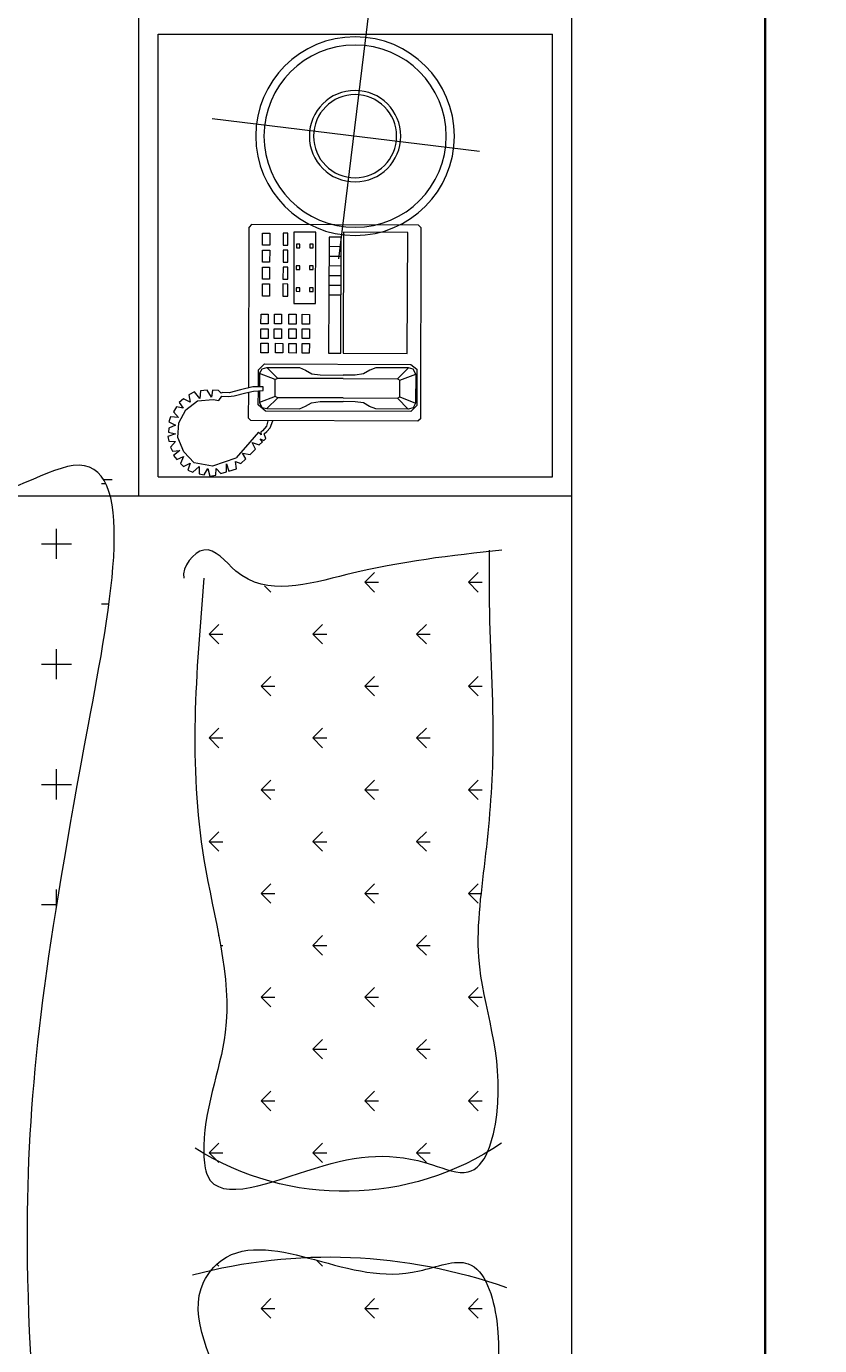
# Model space of a CAD drawing. Units: inches. Extents: x 3731 to 4318, y 1310 to 2388.
# Tile 20 of 57: x 4203 to 4237, y 1445 to 1502. Entities that reach past the tile are written whole.
import ezdxf

# ---------------------------------------------------------------- set-up
doc = ezdxf.new("R2010")
doc.units = ezdxf.units.IN
for name, color, linetype, lineweight in [('A-ANNO-DIMS', 2, 'Continuous', 18), ('A-FURN', 8, 'Continuous', 13), ('A-WALL', 7, 'Continuous', 35)]:
    doc.layers.add(name, color=color, linetype=linetype, lineweight=lineweight)
doc.styles.get("Standard").update_dxf_attribs({"font": 'arial.ttf'})
doc.dimstyles.get("Standard").update_dxf_attribs({"dimtxt": 0.18, "dimasz": 0.18, "dimexe": 0.18, "dimexo": 0.0625, "dimgap": 0.09, "dimtad": 0, "dimtih": 1, "dimtoh": 1, "dimdec": 4, "dimzin": 0, "dimdsep": 46, "dimtxsty": 'Standard', "dimcen": 0.09, "dimadec": 0, "dimazin": 0, "dimtfac": 1, "dimtdec": 4, "dimtofl": 0, "dimtmove": 0, "dimatfit": 3, "dimfxl": 1, "dimtolj": 1, "dimtzin": 0, "dimarcsym": 0})

# ---------------------------------------------------------------- blocks, each defined once
blk = doc.blocks.new('A$C200C7901')
for p, q in [((0.5, 2.3334), (2, 2.3334)), ((2, 2.3334), (2.5, 2.3334)), ((2, 1.6055), (2, 2.3334)), ((1.3176, 2.1721), (1.3075, 2.1822)), ((1.3176, 2.1721), (1.3075, 2.1822)), ((1.206, 2.0681), (1.1997, 2.0744)), ((1.206, 2.0681), (1.1997, 2.0744)), ((1.2019, 1.9645), (1.1997, 1.9666)), ((1.2019, 1.9645), (1.1997, 1.9666)), ((2, 1.8834), (2.5, 1.8834)), ((2.0171, 1.8467), (2.0171, 1.8556)), ((2.0171, 1.8467), (2.0171, 1.8556)), ((2.0129, 1.8445), (2.0129, 1.849)), ((2.0129, 1.8445), (2.0129, 1.849))]:
    blk.add_line(p, q)
at = {"linetype": 'ByBlock'}
for p, q in [((2.02, 2.3134), (2.48, 2.3134)), ((2.02, 1.9034), (2.02, 2.3134)), ((2.48, 1.9034), (2.48, 2.3134)), ((1.1559, 2.2259), (1.1458, 2.236)), ((1.1559, 2.2259), (1.1458, 2.236)), ((1.1559, 2.2259), (1.1559, 2.2402)), ((1.1559, 2.2259), (1.1559, 2.2402)), ((1.1559, 2.2259), (1.166, 2.236)), ((1.1559, 2.2259), (1.166, 2.236)), ((1.3714, 2.2259), (1.3613, 2.236)), ((1.3714, 2.2259), (1.3613, 2.236)), ((1.3714, 2.2259), (1.3714, 2.2402)), ((1.3714, 2.2259), (1.3714, 2.2402)), ((1.3714, 2.2259), (1.3815, 2.236)), ((1.3714, 2.2259), (1.3815, 2.236)), ((1.4792, 2.2259), (1.4691, 2.236)), ((1.4792, 2.2259), (1.4691, 2.236)), ((1.4792, 2.2259), (1.4792, 2.2402)), ((1.4792, 2.2259), (1.4792, 2.2402)), ((1.4792, 2.2259), (1.4893, 2.236)), ((1.4792, 2.2259), (1.4893, 2.236)), ((1.587, 2.2259), (1.5769, 2.236)), ((1.587, 2.2259), (1.5769, 2.236)), ((1.587, 2.2259), (1.587, 2.2393)), ((1.587, 2.2259), (1.587, 2.2393)), ((1.587, 2.2259), (1.5971, 2.236)), ((1.587, 2.2259), (1.5971, 2.236)), ((1.6947, 2.2259), (1.6846, 2.236)), ((1.6947, 2.2259), (1.6846, 2.236)), ((1.6947, 2.2259), (1.6947, 2.2402)), ((1.6947, 2.2259), (1.6947, 2.2402)), ((1.6947, 2.2259), (1.7048, 2.236)), ((1.6947, 2.2259), (1.7048, 2.236)), ((1.8025, 2.2259), (1.7924, 2.236)), ((1.8025, 2.2259), (1.7924, 2.236)), ((1.8025, 2.2259), (1.8025, 2.2402)), ((1.8025, 2.2259), (1.8025, 2.2402)), ((1.8025, 2.2259), (1.8126, 2.236)), ((1.8025, 2.2259), (1.8126, 2.236)), ((1.9103, 2.2259), (1.9002, 2.236)), ((1.9103, 2.2259), (1.9002, 2.236)), ((1.9103, 2.2259), (1.9103, 2.2402)), ((1.9103, 2.2259), (1.9103, 2.2402)), ((1.9103, 2.2259), (1.9204, 2.236)), ((1.9103, 2.2259), (1.9204, 2.236)), ((2.3581, 2.2373), (2.3919, 1.9595)), ((1.3176, 2.172), (1.3176, 2.1863)), ((1.3176, 2.172), (1.3176, 2.1863)), ((1.3176, 2.1721), (1.3277, 2.1822)), ((1.3176, 2.1721), (1.3277, 2.1822)), ((1.4253, 2.1721), (1.4152, 2.1822)), ((1.4253, 2.1721), (1.4152, 2.1822)), ((1.4253, 2.172), (1.4253, 2.1863)), ((1.4253, 2.172), (1.4253, 2.1863)), ((1.4253, 2.1721), (1.4354, 2.1822)), ((1.4253, 2.1721), (1.4354, 2.1822)), ((1.5331, 2.1721), (1.523, 2.1822)), ((1.5331, 2.1721), (1.523, 2.1822)), ((1.5331, 2.172), (1.5331, 2.1863)), ((1.5331, 2.172), (1.5331, 2.1863)), ((1.5331, 2.1721), (1.5432, 2.1822)), ((1.5331, 2.1721), (1.5432, 2.1822)), ((1.6409, 2.1721), (1.6308, 2.1822)), ((1.6409, 2.1721), (1.6308, 2.1822)), ((1.6408, 2.172), (1.6408, 2.1863)), ((1.6408, 2.172), (1.6408, 2.1863)), ((1.6409, 2.1721), (1.651, 2.1822)), ((1.6409, 2.1721), (1.651, 2.1822)), ((1.7486, 2.1721), (1.7385, 2.1822)), ((1.7486, 2.1721), (1.7385, 2.1822)), ((1.7486, 2.172), (1.7486, 2.1863)), ((1.7486, 2.172), (1.7486, 2.1863)), ((1.7486, 2.1721), (1.7587, 2.1822)), ((1.7486, 2.1721), (1.7587, 2.1822)), ((1.8564, 2.1721), (1.8463, 2.1822)), ((1.8564, 2.1721), (1.8463, 2.1822)), ((1.8564, 2.172), (1.8564, 2.1863)), ((1.8564, 2.172), (1.8564, 2.1863)), ((1.8564, 2.1721), (1.8665, 2.1822)), ((1.8564, 2.1721), (1.8665, 2.1822)), ((2.0802, 2.176), (2.0777, 2.1734)), ((2.0777, 2.1734), (2.0783, 1.9999)), ((2.2789, 2.1766), (2.0802, 2.176)), ((2.0941, 2.1722), (2.0878, 2.1659)), ((2.0878, 2.1659), (2.0883, 2.015)), ((2.0915, 2.1685), (2.0903, 2.1634)), ((2.0966, 2.171), (2.0915, 2.1685)), ((2.1318, 2.1724), (2.0941, 2.1722)), ((2.1267, 2.1711), (2.0966, 2.171)), ((2.1029, 2.1547), (2.0966, 2.171)), ((2.1205, 2.1547), (2.1267, 2.1711)), ((2.1267, 2.1711), (2.1318, 2.1686)), ((2.1368, 2.1661), (2.1318, 2.1724)), ((2.1318, 2.1686), (2.1331, 2.1636)), ((2.1373, 2.014), (2.1368, 2.1661)), ((2.2789, 2.1766), (2.2814, 2.1741)), ((2.2814, 2.1741), (2.282, 2.0006)), ((2.0903, 2.1634), (2.1017, 2.1521)), ((2.0903, 2.1634), (2.0904, 2.1295)), ((2.1017, 2.1521), (2.1029, 2.1547)), ((2.1019, 2.0956), (2.1017, 2.1521)), ((2.1029, 2.1547), (2.1205, 2.1547)), ((2.1218, 2.1522), (2.1205, 2.1547)), ((2.1331, 2.1636), (2.1218, 2.1522)), ((2.122, 2.0956), (2.1218, 2.1522)), ((2.1331, 2.1636), (2.1332, 2.1296)), ((2.1481, 2.1624), (2.2739, 2.1628)), ((2.1484, 2.0957), (2.1481, 2.1624)), ((2.2739, 2.1628), (2.2741, 2.0961)), ((1.1559, 2.1182), (1.1458, 2.1283)), ((1.1559, 2.1182), (1.1458, 2.1283)), ((1.1559, 2.1182), (1.1559, 2.1325)), ((1.1559, 2.1182), (1.1559, 2.1325)), ((1.1559, 2.1182), (1.166, 2.1283)), ((1.1559, 2.1182), (1.166, 2.1283)), ((1.3714, 2.1182), (1.3613, 2.1283)), ((1.3714, 2.1182), (1.3613, 2.1283)), ((1.3714, 2.1182), (1.3714, 2.1325)), ((1.3714, 2.1182), (1.3714, 2.1325)), ((1.3714, 2.1182), (1.3815, 2.1283)), ((1.3714, 2.1182), (1.3815, 2.1283)), ((1.4792, 2.1182), (1.4691, 2.1283)), ((1.4792, 2.1182), (1.4691, 2.1283)), ((1.4792, 2.1182), (1.4792, 2.1325)), ((1.4792, 2.1182), (1.4792, 2.1325)), ((1.4792, 2.1182), (1.4893, 2.1283)), ((1.4792, 2.1182), (1.4893, 2.1283)), ((1.587, 2.1182), (1.5769, 2.1283)), ((1.587, 2.1182), (1.5769, 2.1283)), ((1.587, 2.1182), (1.587, 2.1325)), ((1.587, 2.1182), (1.587, 2.1325)), ((1.587, 2.1182), (1.5971, 2.1283)), ((1.587, 2.1182), (1.5971, 2.1283)), ((1.6947, 2.1182), (1.6846, 2.1283)), ((1.6947, 2.1182), (1.6846, 2.1283)), ((1.6947, 2.1182), (1.6947, 2.1325)), ((1.6947, 2.1182), (1.6947, 2.1325)), ((1.6947, 2.1182), (1.7048, 2.1283)), ((1.6947, 2.1182), (1.7048, 2.1283)), ((1.8025, 2.1182), (1.7924, 2.1283)), ((1.8025, 2.1182), (1.7924, 2.1283)), ((1.8025, 2.1182), (1.8025, 2.1325)), ((1.8025, 2.1182), (1.8025, 2.1325)), ((1.8025, 2.1182), (1.8126, 2.1283)), ((1.8025, 2.1182), (1.8126, 2.1283)), ((1.9103, 2.1182), (1.9002, 2.1283)), ((1.9103, 2.1182), (1.9002, 2.1283)), ((1.9103, 2.1182), (1.9103, 2.1325)), ((1.9103, 2.1182), (1.9103, 2.1325)), ((1.9103, 2.1182), (1.9204, 2.1283)), ((1.9103, 2.1182), (1.9204, 2.1283)), ((2.0904, 2.1295), (2.093, 2.1232)), ((2.1332, 2.1296), (2.1307, 2.1233)), ((2.093, 2.1232), (2.0968, 2.1169)), ((2.0968, 2.1169), (2.098, 2.1081)), ((2.1269, 2.117), (2.1257, 2.1082)), ((2.1307, 2.1233), (2.1269, 2.117)), ((2.2464, 2.0911), (2.5044, 2.1228)), ((2.098, 2.1081), (2.0981, 2.0956)), ((2.1257, 2.1082), (2.1257, 2.0956)), ((2.0982, 2.0717), (2.0981, 2.0956)), ((2.1019, 2.0956), (2.1021, 2.0277)), ((2.122, 2.0956), (2.1222, 2.0277)), ((2.1258, 2.0718), (2.1257, 2.0956)), ((2.2741, 2.0961), (2.1484, 2.0957)), ((2.1484, 2.0932), (2.2691, 2.0936)), ((2.1484, 2.0806), (2.1484, 2.0932)), ((2.2087, 2.0934), (2.2088, 2.0808)), ((2.2188, 2.0934), (2.2188, 2.0809)), ((2.2288, 2.0935), (2.2289, 2.0809)), ((2.2389, 2.0935), (2.239, 2.0809)), ((2.249, 2.0935), (2.249, 2.081)), ((2.259, 2.0936), (2.2591, 2.081)), ((2.2691, 2.0936), (2.2691, 2.081)), ((1.3176, 2.0643), (1.3075, 2.0744)), ((1.3176, 2.0643), (1.3075, 2.0744)), ((1.3176, 2.0643), (1.3176, 2.0786)), ((1.3176, 2.0643), (1.3176, 2.0786)), ((1.3176, 2.0643), (1.3277, 2.0744)), ((1.3176, 2.0643), (1.3277, 2.0744)), ((1.4253, 2.0643), (1.4152, 2.0744)), ((1.4253, 2.0643), (1.4152, 2.0744)), ((1.4253, 2.0643), (1.4253, 2.0786)), ((1.4253, 2.0643), (1.4253, 2.0786)), ((1.4253, 2.0643), (1.4354, 2.0744)), ((1.4253, 2.0643), (1.4354, 2.0744)), ((1.5331, 2.0643), (1.523, 2.0744)), ((1.5331, 2.0643), (1.523, 2.0744)), ((1.5331, 2.0643), (1.5331, 2.0786)), ((1.5331, 2.0643), (1.5331, 2.0786)), ((1.5331, 2.0643), (1.5432, 2.0744)), ((1.5331, 2.0643), (1.5432, 2.0744)), ((1.6409, 2.0643), (1.6308, 2.0744)), ((1.6409, 2.0643), (1.6308, 2.0744)), ((1.6408, 2.0643), (1.6408, 2.0786)), ((1.6408, 2.0643), (1.6408, 2.0786)), ((1.6409, 2.0643), (1.651, 2.0744)), ((1.6409, 2.0643), (1.651, 2.0744)), ((1.7486, 2.0643), (1.7385, 2.0744)), ((1.7486, 2.0643), (1.7385, 2.0744)), ((1.7486, 2.0643), (1.7486, 2.0786)), ((1.7486, 2.0643), (1.7486, 2.0786)), ((1.7486, 2.0643), (1.7587, 2.0744)), ((1.7486, 2.0643), (1.7587, 2.0744)), ((1.8564, 2.0643), (1.8463, 2.0744)), ((1.8564, 2.0643), (1.8463, 2.0744)), ((1.8564, 2.0643), (1.8564, 2.0786)), ((1.8564, 2.0643), (1.8564, 2.0786)), ((1.8564, 2.0643), (1.8665, 2.0744)), ((1.8564, 2.0643), (1.8665, 2.0744)), ((2.0969, 2.0629), (2.0982, 2.0717)), ((2.1271, 2.063), (2.1258, 2.0718)), ((2.2691, 2.081), (2.1484, 2.0806)), ((2.0907, 2.0503), (2.0932, 2.0566)), ((2.0932, 2.0566), (2.0969, 2.0629)), ((2.1309, 2.0567), (2.1271, 2.063)), ((2.1334, 2.0504), (2.1309, 2.0567)), ((2.1586, 2.0606), (2.1485, 2.0605)), ((2.1485, 2.0605), (2.1485, 2.053)), ((2.1586, 2.053), (2.1586, 2.0606)), ((2.1636, 2.0606), (2.1636, 2.053)), ((2.1736, 2.0606), (2.1636, 2.0606)), ((2.1737, 2.0531), (2.1736, 2.0606)), ((2.1887, 2.0607), (2.1787, 2.0606)), ((2.1787, 2.0606), (2.1787, 2.0531)), ((2.1888, 2.0531), (2.1887, 2.0607)), ((2.2, 2.067), (2.2742, 2.0672)), ((2.2001, 2.0443), (2.2, 2.067)), ((2.2126, 2.0645), (2.2164, 2.0645)), ((2.2126, 2.0607), (2.2126, 2.0645)), ((2.2164, 2.0607), (2.2126, 2.0607)), ((2.2164, 2.0645), (2.2164, 2.0607)), ((2.2352, 2.0646), (2.239, 2.0646)), ((2.2352, 2.0608), (2.2352, 2.0646)), ((2.239, 2.0608), (2.2352, 2.0608)), ((2.239, 2.0646), (2.239, 2.0608)), ((2.2579, 2.0609), (2.2579, 2.0647)), ((2.2579, 2.0647), (2.2616, 2.0647)), ((2.2616, 2.0609), (2.2579, 2.0609)), ((2.2616, 2.0647), (2.2616, 2.0609)), ((2.2742, 2.0672), (2.2743, 2.0446)), ((2.0908, 2.0163), (2.0907, 2.0503)), ((2.1336, 2.0165), (2.1334, 2.0504)), ((2.1485, 2.053), (2.1586, 2.053)), ((2.1485, 2.0467), (2.1486, 2.0391)), ((2.1586, 2.0467), (2.1485, 2.0467)), ((2.1586, 2.0392), (2.1586, 2.0467)), ((2.1636, 2.053), (2.1737, 2.0531)), ((2.1737, 2.0468), (2.1636, 2.0467)), ((2.1636, 2.0467), (2.1637, 2.0392)), ((2.1737, 2.0392), (2.1737, 2.0468)), ((2.1787, 2.0531), (2.1888, 2.0531)), ((2.1787, 2.0468), (2.1787, 2.0392)), ((2.1888, 2.0468), (2.1787, 2.0468)), ((2.1888, 2.0393), (2.1888, 2.0468)), ((2.2743, 2.0446), (2.2001, 2.0443)), ((2.2126, 2.0507), (2.2164, 2.0507)), ((2.2127, 2.0469), (2.2126, 2.0507)), ((2.2164, 2.0469), (2.2127, 2.0469)), ((2.2164, 2.0507), (2.2164, 2.0469)), ((2.2353, 2.0508), (2.2391, 2.0508)), ((2.2353, 2.047), (2.2353, 2.0508)), ((2.2391, 2.047), (2.2353, 2.047)), ((2.2391, 2.0508), (2.2391, 2.047)), ((2.2579, 2.0508), (2.2617, 2.0508)), ((2.2579, 2.0471), (2.2579, 2.0508)), ((2.2617, 2.0471), (2.2579, 2.0471)), ((2.2617, 2.0508), (2.2617, 2.0471)), ((2.1486, 2.0391), (2.1586, 2.0392)), ((2.1586, 2.0329), (2.1486, 2.0329)), ((2.1486, 2.0329), (2.1486, 2.0253)), ((2.1587, 2.0253), (2.1586, 2.0329)), ((2.1637, 2.0392), (2.1737, 2.0392)), ((2.1637, 2.0317), (2.1637, 2.0241)), ((2.1737, 2.0317), (2.1637, 2.0317)), ((2.1738, 2.0241), (2.1737, 2.0317)), ((2.1787, 2.0392), (2.1888, 2.0393)), ((2.1788, 2.0317), (2.1788, 2.0242)), ((2.1888, 2.0317), (2.1788, 2.0317)), ((2.1889, 2.0242), (2.1888, 2.0317)), ((2.2077, 2.0331), (2.2077, 2.0381)), ((2.2077, 2.0381), (2.2202, 2.0381)), ((2.2203, 2.0331), (2.2077, 2.0331)), ((2.2202, 2.0381), (2.2203, 2.0331)), ((2.2253, 2.0381), (2.2378, 2.0382)), ((2.2253, 2.0331), (2.2253, 2.0381)), ((2.2379, 2.0332), (2.2253, 2.0331)), ((2.2378, 2.0382), (2.2379, 2.0332)), ((2.2429, 2.0332), (2.2429, 2.0382)), ((2.2429, 2.0382), (2.2554, 2.0382)), ((2.2555, 2.0332), (2.2429, 2.0332)), ((2.2554, 2.0382), (2.2555, 2.0332)), ((2.2605, 2.0332), (2.2605, 2.0383)), ((2.2605, 2.0383), (2.273, 2.0383)), ((2.2731, 2.0333), (2.2605, 2.0332)), ((2.273, 2.0383), (2.2731, 2.0333)), ((1.1559, 2.0104), (1.1458, 2.0205)), ((1.1559, 2.0104), (1.1458, 2.0205)), ((1.1559, 2.0104), (1.1559, 2.0247)), ((1.1559, 2.0104), (1.1559, 2.0247)), ((1.1559, 2.0104), (1.166, 2.0205)), ((1.1559, 2.0104), (1.166, 2.0205)), ((1.3714, 2.0104), (1.3613, 2.0205)), ((1.3714, 2.0104), (1.3613, 2.0205)), ((1.3714, 2.0104), (1.3714, 2.0247)), ((1.3714, 2.0104), (1.3714, 2.0247)), ((1.3714, 2.0104), (1.3815, 2.0205)), ((1.3714, 2.0104), (1.3815, 2.0205)), ((1.4792, 2.0104), (1.4691, 2.0205)), ((1.4792, 2.0104), (1.4691, 2.0205)), ((1.4792, 2.0104), (1.4792, 2.0247)), ((1.4792, 2.0104), (1.4792, 2.0247)), ((1.4792, 2.0104), (1.4893, 2.0205)), ((1.4792, 2.0104), (1.4893, 2.0205)), ((1.587, 2.0104), (1.5769, 2.0205)), ((1.587, 2.0104), (1.5769, 2.0205)), ((1.587, 2.0104), (1.587, 2.0247)), ((1.587, 2.0104), (1.587, 2.0247)), ((1.587, 2.0104), (1.5971, 2.0205)), ((1.587, 2.0104), (1.5971, 2.0205)), ((1.6947, 2.0104), (1.6846, 2.0205)), ((1.6947, 2.0104), (1.6846, 2.0205)), ((1.6947, 2.0104), (1.6947, 2.0247)), ((1.6947, 2.0104), (1.6947, 2.0247)), ((1.6947, 2.0104), (1.7048, 2.0205)), ((1.6947, 2.0104), (1.7048, 2.0205)), ((1.8025, 2.0104), (1.7924, 2.0205)), ((1.8025, 2.0104), (1.7924, 2.0205)), ((1.8025, 2.0104), (1.8025, 2.0247)), ((1.8025, 2.0104), (1.8025, 2.0247)), ((1.8025, 2.0104), (1.8126, 2.0205)), ((1.8025, 2.0104), (1.8126, 2.0205)), ((1.9068, 2.0139), (1.9002, 2.0205)), ((1.9068, 2.0139), (1.9002, 2.0205)), ((2.0576, 2.0133), (2.0598, 2.0155)), ((2.0598, 2.0155), (2.0645, 2.0137)), ((2.0645, 2.0137), (2.0671, 2.0162)), ((2.0671, 2.0162), (2.0707, 2.0197)), ((2.0727, 2.016), (2.0676, 2.012)), ((2.0707, 2.0197), (2.0782, 2.0226)), ((2.0782, 2.0175), (2.0727, 2.016)), ((2.0883, 2.015), (2.0946, 2.0075)), ((2.0908, 2.0163), (2.1021, 2.0277)), ((2.0921, 2.0113), (2.0908, 2.0163)), ((2.1034, 2.0252), (2.0971, 2.0088)), ((2.1021, 2.0277), (2.1034, 2.0252)), ((2.1034, 2.0252), (2.121, 2.0252)), ((2.1222, 2.0277), (2.121, 2.0252)), ((2.121, 2.0252), (2.1273, 2.0089)), ((2.1336, 2.0165), (2.1222, 2.0277)), ((2.1323, 2.0114), (2.1336, 2.0165)), ((2.1486, 2.0253), (2.1587, 2.0253)), ((2.1587, 2.0178), (2.1486, 2.0178)), ((2.1486, 2.0178), (2.1487, 2.0102)), ((2.1587, 2.0103), (2.1587, 2.0178)), ((2.1637, 2.0241), (2.1738, 2.0241)), ((2.1738, 2.0179), (2.1637, 2.0178)), ((2.1637, 2.0178), (2.1638, 2.0103)), ((2.1738, 2.0103), (2.1738, 2.0179)), ((2.1788, 2.0242), (2.1889, 2.0242)), ((2.1788, 2.0179), (2.1788, 2.0103)), ((2.1889, 2.0179), (2.1788, 2.0179)), ((2.1889, 2.0104), (2.1889, 2.0179)), ((2.2203, 2.0193), (2.2077, 2.0192)), ((2.2077, 2.0192), (2.2078, 2.0117)), ((2.2203, 2.0117), (2.2203, 2.0193)), ((2.2379, 2.0193), (2.2253, 2.0193)), ((2.2253, 2.0193), (2.2254, 2.0117)), ((2.2379, 2.0118), (2.2379, 2.0193)), ((2.2555, 2.0194), (2.2429, 2.0193)), ((2.2429, 2.0193), (2.243, 2.0118)), ((2.2555, 2.0118), (2.2555, 2.0194)), ((2.2605, 2.0194), (2.2606, 2.0119)), ((2.2731, 2.0194), (2.2605, 2.0194)), ((2.2731, 2.0119), (2.2731, 2.0194)), ((2.0431, 1.999), (2.0488, 2.0046)), ((2.0488, 2.0046), (2.0557, 2.0011)), ((2.053, 2.0084), (2.0563, 2.0119)), ((2.0557, 2.0011), (2.053, 2.0084)), ((2.0663, 2.0077), (2.0561, 1.9986)), ((2.0563, 2.0119), (2.0594, 2.0095)), ((2.0594, 2.0095), (2.0576, 2.0133)), ((2.0663, 2.0102), (2.0636, 2.0104)), ((2.0636, 2.0104), (2.0663, 2.0077)), ((2.0676, 2.012), (2.0663, 2.0102)), ((2.0971, 2.0088), (2.0921, 2.0113)), ((2.0946, 2.0075), (2.1093, 2.0076)), ((2.1094, 2.0088), (2.0971, 2.0088)), ((2.1072, 1.9944), (2.109, 2.0025)), ((2.109, 2.0025), (2.1097, 2.0126)), ((2.1097, 2.0126), (2.1135, 2.0126)), ((2.1133, 2.0018), (2.1103, 1.989)), ((2.1135, 2.0126), (2.1133, 2.0018)), ((2.1273, 2.0089), (2.1134, 2.0088)), ((2.1134, 2.0076), (2.1311, 2.0077)), ((2.1273, 2.0089), (2.1323, 2.0114)), ((2.1311, 2.0077), (2.1373, 2.014)), ((2.1487, 2.0102), (2.1587, 2.0103)), ((2.1638, 2.0103), (2.1738, 2.0103)), ((2.1788, 2.0103), (2.1889, 2.0104)), ((2.2078, 2.0117), (2.2203, 2.0117)), ((2.2254, 2.0117), (2.2379, 2.0118)), ((2.243, 2.0118), (2.2555, 2.0118)), ((2.2606, 2.0119), (2.2731, 2.0119)), ((2.0338, 1.9895), (2.0386, 1.9946)), ((2.0358, 1.9839), (2.0338, 1.9895)), ((2.0386, 1.9946), (2.0444, 1.9911)), ((2.0561, 1.9986), (2.0396, 1.9844)), ((2.0444, 1.9911), (2.0431, 1.999)), ((2.0783, 1.9999), (2.0808, 1.9974)), ((2.0808, 1.9974), (2.1079, 1.9975)), ((2.1042, 1.9824), (2.1072, 1.9944)), ((2.1103, 1.989), (2.1073, 1.9771)), ((2.1123, 1.9975), (2.2795, 1.9981)), ((2.282, 2.0006), (2.2795, 1.9981)), ((2.0234, 1.9686), (2.0251, 1.9745)), ((2.0251, 1.9745), (2.0333, 1.9743)), ((2.0259, 1.977), (2.0281, 1.9847)), ((2.0333, 1.9743), (2.0259, 1.977)), ((2.0281, 1.9847), (2.0358, 1.9839)), ((2.0393, 1.984), (2.031, 1.96)), ((2.1035, 1.9763), (2.1042, 1.9824)), ((2.1038, 1.9697), (2.1035, 1.9763)), ((2.1073, 1.9771), (2.1076, 1.9704)), ((1.3176, 1.9565), (1.3075, 1.9666)), ((1.3176, 1.9565), (1.3075, 1.9666)), ((1.3176, 1.9565), (1.3176, 1.9708)), ((1.3176, 1.9565), (1.3176, 1.9708)), ((1.3176, 1.9565), (1.3277, 1.9666)), ((1.3176, 1.9565), (1.3277, 1.9666)), ((1.4253, 1.9703), (1.4253, 1.9708)), ((1.4253, 1.9703), (1.4253, 1.9708)), ((1.5331, 1.9683), (1.5331, 1.9708)), ((1.5331, 1.9683), (1.5331, 1.9708)), ((1.543, 1.9665), (1.5432, 1.9666)), ((1.543, 1.9665), (1.5432, 1.9666)), ((1.6409, 1.9565), (1.6308, 1.9666)), ((1.6409, 1.9565), (1.6308, 1.9666)), ((1.6408, 1.9565), (1.6408, 1.9708)), ((1.6408, 1.9565), (1.6408, 1.9708)), ((1.6409, 1.9565), (1.651, 1.9666)), ((1.6409, 1.9565), (1.651, 1.9666)), ((1.7486, 1.9565), (1.7385, 1.9666)), ((1.7486, 1.9565), (1.7385, 1.9666)), ((1.7486, 1.9565), (1.7486, 1.9708)), ((1.7486, 1.9565), (1.7486, 1.9708)), ((1.7486, 1.9565), (1.7587, 1.9666)), ((1.7486, 1.9565), (1.7587, 1.9666)), ((1.8564, 1.9565), (1.8463, 1.9666)), ((1.8564, 1.9565), (1.8463, 1.9666)), ((1.8564, 1.9565), (1.8564, 1.9708)), ((1.8564, 1.9565), (1.8564, 1.9708)), ((1.8564, 1.9565), (1.8665, 1.9666)), ((1.8564, 1.9565), (1.8665, 1.9666)), ((2.0206, 1.9572), (2.0218, 1.9635)), ((2.0218, 1.9635), (2.0287, 1.9636)), ((2.0287, 1.9636), (2.0234, 1.9686)), ((2.099, 1.9444), (2.1002, 1.9605)), ((2.0992, 1.9663), (2.1038, 1.9697)), ((2.1002, 1.9605), (2.0992, 1.9663)), ((2.1076, 1.9704), (2.1068, 1.9689)), ((2.1068, 1.9689), (2.1096, 1.9661)), ((2.1096, 1.9661), (2.1101, 1.96)), ((2.0285, 1.9549), (2.0206, 1.9572)), ((2.0219, 1.9511), (2.0285, 1.9549)), ((2.0229, 1.946), (2.0219, 1.9511)), ((2.031, 1.96), (2.0346, 1.9409)), ((2.1094, 1.9475), (2.1013, 1.9467)), ((2.1013, 1.9467), (2.1084, 1.9412)), ((2.1101, 1.96), (2.1028, 1.9587)), ((2.1028, 1.9587), (2.1099, 1.9544)), ((2.1099, 1.9544), (2.1094, 1.9475)), ((2.0308, 1.9462), (2.0229, 1.946)), ((2.0247, 1.9394), (2.0308, 1.9462)), ((2.0268, 1.9343), (2.0247, 1.9394)), ((2.0341, 1.9366), (2.0268, 1.9343)), ((2.0306, 1.9297), (2.0341, 1.9366)), ((2.0346, 1.9409), (2.0459, 1.93)), ((2.0894, 1.9322), (2.099, 1.9444)), ((2.1051, 1.9353), (2.0975, 1.9368)), ((2.0975, 1.9368), (2.1011, 1.9297)), ((2.1084, 1.9412), (2.1051, 1.9353)), ((2.0339, 1.9267), (2.0306, 1.9297)), ((2.041, 1.9297), (2.0339, 1.9267)), ((2.038, 1.9228), (2.041, 1.9297)), ((2.0421, 1.9193), (2.038, 1.9228)), ((2.0474, 1.9259), (2.0421, 1.9193)), ((2.0459, 1.93), (2.0607, 1.9237)), ((2.0467, 1.9183), (2.0474, 1.9259)), ((2.0566, 1.9214), (2.0508, 1.9163)), ((2.0569, 1.9145), (2.0566, 1.9214)), ((2.0607, 1.9237), (2.0759, 1.925)), ((2.0645, 1.9214), (2.0617, 1.9133)), ((2.0663, 1.914), (2.0645, 1.9214)), ((2.0736, 1.9214), (2.0706, 1.9146)), ((2.077, 1.9146), (2.0736, 1.9214)), ((2.0759, 1.925), (2.0894, 1.9322)), ((2.0876, 1.9195), (2.0815, 1.9245)), ((2.0815, 1.9245), (2.0823, 1.9161)), ((2.0925, 1.9225), (2.0876, 1.9195)), ((2.0973, 1.9251), (2.0914, 1.9294)), ((2.0914, 1.9294), (2.0925, 1.9225)), ((2.1011, 1.9297), (2.0973, 1.9251)), ((2.0508, 1.9163), (2.0467, 1.9183)), ((2.0617, 1.9133), (2.0569, 1.9145)), ((2.0706, 1.9146), (2.0663, 1.914)), ((2.0823, 1.9161), (2.077, 1.9146)), ((2.02, 1.9034), (2.48, 1.9034)), ((1.8879, 1.8445), (1.8879, 1.8523)), ((1.8879, 1.8445), (1.8879, 1.8523)), ((1.7004, 1.782), (1.7004, 1.8133)), ((1.7004, 1.782), (1.7004, 1.8133)), ((1.8254, 1.782), (1.8254, 1.8133)), ((1.8254, 1.782), (1.8254, 1.8133)), ((1.9504, 1.782), (1.9504, 1.8133)), ((1.9504, 1.782), (1.9504, 1.8133)), ((1.573, 1.7977), (1.591, 1.7977)), ((1.573, 1.7977), (1.591, 1.7977)), ((1.5754, 1.782), (1.5754, 1.7981)), ((1.5754, 1.782), (1.5754, 1.7981)), ((1.6847, 1.7977), (1.716, 1.7977)), ((1.6847, 1.7977), (1.716, 1.7977)), ((1.8097, 1.7977), (1.841, 1.7977)), ((1.8097, 1.7977), (1.841, 1.7977)), ((1.9347, 1.7977), (1.966, 1.7977)), ((1.9347, 1.7977), (1.966, 1.7977))]:
    blk.add_line(p, q, dxfattribs=at)
for radius in [0.1032, 0.0947, 0.0475, 0.0432]:
    blk.add_circle((2.3739, 2.1081), radius, dxfattribs=at)
for centre, radius, start, end in [((0.658, 2.0811), 0.5513, 345.0722, 19.5492), ((1.5685, 2.097), 0.291, 145.8603, 212.2445)]:
    blk.add_arc(centre, radius, start, end)
for points, knots in [([(0.5854, 1.951), (0.6835, 1.9407), (0.8425, 1.9242), (1.0374, 2.0054), (1.1564, 1.9255), (1.2274, 1.9841), (1.2052, 2.0751), (1.1815, 2.152), (1.2176, 2.2368), (1.0992, 2.2731), (1.0008, 2.2255), (0.8698, 2.246), (0.7481, 2.2548), (0.6426, 2.2473), (0.5746, 2.2478), (0.5562, 2.2479)], [0, 0, 0, 0, 292.165466, 473.33038, 601.631673, 630.723769, 727.138505, 836.819956, 887.958136, 954.42438, 1118.989809, 1227.016542, 1338.750986, 1487.447361, 1542.751028, 1542.751028, 1542.751028, 1542.751028]), ([(1.9146, 1.951), (1.8174, 1.9428), (1.6601, 1.9297), (1.4574, 1.9942), (1.3549, 1.9462), (1.2593, 1.9563), (1.314, 2.0834), (1.3193, 2.1569), (1.2853, 2.2393), (1.4031, 2.2724), (1.4987, 2.2256), (1.6304, 2.2459), (1.7519, 2.2548), (1.8574, 2.2473), (1.9254, 2.2478), (1.9438, 2.2479)], [0, 0, 0, 0, 292.165466, 473.33038, 601.631673, 624.236147, 735.870502, 858.452188, 896.317728, 962.783971, 1127.3494, 1235.376134, 1347.110578, 1495.806953, 1551.11062, 1551.11062, 1551.11062, 1551.11062]), ([(1.9438, 2.2608), (1.9381, 2.2086), (1.9282, 2.1195), (1.8897, 2.0022), (1.9591, 1.9538), (1.9264, 1.9278), (1.9146, 1.93)], [0, 0, 0, 0, 163.411291, 278.570782, 318.445997, 354.484131, 354.484131, 354.484131, 354.484131]), ([(0.4485, 1.7835), (0.4321, 1.7496), (0.4062, 1.6964), (0.49, 1.6713), (0.4719, 1.5969), (0.4123, 1.592), (0.4233, 1.5337), (0.4954, 1.5086), (0.4012, 1.4738), (0.3253, 1.4306), (0.4113, 1.3764), (0.3688, 1.3065), (0.5579, 1.2663), (0.741, 1.4533), (1.1127, 1.1109), (1.4811, 1.2478), (1.7885, 1.3492), (2.0357, 1.1637), (2.0748, 1.2974), (2.0876, 1.349), (2.0192, 1.3805), (2.0564, 1.4298), (2.0588, 1.4846), (1.9759, 1.5349), (2.1004, 1.5845), (2.0397, 1.6519), (1.971, 1.7053), (2.1104, 1.8981), (1.5946, 1.7967), (1.2448, 1.7472), (0.8129, 1.7935), (0.4953, 1.8548), (0.4582, 1.7983), (0.4485, 1.7835)], [0, 0, 0, 0, 88.420092, 139.08588, 204.302936, 239.695496, 287.801042, 327.365471, 412.960499, 463.626286, 552.059846, 584.668336, 662.614915, 940.993281, 1309.926334, 1844.022653, 1996.276242, 2316.43048, 2341.441004, 2404.707416, 2449.463774, 2514.680778, 2538.40571, 2613.031547, 2697.13096, 2760.903931, 2822.692699, 2945.47, 3215.060018, 3725.584917, 4361.974444, 4504.671998, 4555.32777, 4555.32777, 4555.32777, 4555.32777])]:
    blk.add_open_spline(points, degree=3, knots=knots)
blk = doc.blocks.new('*D32')
at = {"layer": 'A-ANNO-DIMS', "color": 0, "lineweight": -2, "transparency": 16777216}
for p, q in [((4269.211, 1592.319), (4269.211, 1310.251)), ((3835.209, 1359.319), (3835.209, 1310.251)), ((3835.389, 1310.431), (4051.918, 1310.431)), ((4269.031, 1310.431), (4052.502, 1310.431))]:
    blk.add_line(p, q, dxfattribs=at)
at = {"layer": 'A-ANNO-DIMS', "color": 0, "transparency": 16777216}
for points in [[(3835.389, 1310.461), (3835.389, 1310.401), (3835.209, 1310.431)], [(4269.031, 1310.461), (4269.031, 1310.401), (4269.211, 1310.431)]]:
    blk.add_solid(points, dxfattribs=at)
at = {"layer": 'Defpoints', "color": 0, "transparency": 16777216}
for p in [(4269.211, 1592.382), (3835.209, 1359.382), (4269.211, 1310.431)]:
    blk.add_point(p, dxfattribs=at)
at = {"layer": 'A-ANNO-DIMS', "color": 0, "transparency": 16777216, "insert": (4052.21, 1310.431), "char_height": 0.18, "attachment_point": 5}
blk.add_mtext('\\A1;434', dxfattribs=at)
blk = doc.blocks.new('*D47')
at = {"layer": 'A-ANNO-DIMS', "color": 0, "lineweight": -2, "transparency": 16777216}
for p, q in [((4192.209, 1854.319), (4192.209, 1310.251)), ((4234.209, 1854.319), (4234.209, 1310.251)), ((4192.389, 1310.431), (4212.987, 1310.431)), ((4234.029, 1310.431), (4213.43, 1310.431))]:
    blk.add_line(p, q, dxfattribs=at)
at = {"layer": 'A-ANNO-DIMS', "color": 0, "transparency": 16777216}
for points in [[(4192.389, 1310.461), (4192.389, 1310.401), (4192.209, 1310.431)], [(4234.029, 1310.461), (4234.029, 1310.401), (4234.209, 1310.431)]]:
    blk.add_solid(points, dxfattribs=at)
at = {"layer": 'Defpoints', "color": 0, "transparency": 16777216}
for p in [(4192.209, 1854.382), (4234.209, 1854.382), (4234.209, 1310.431)]:
    blk.add_point(p, dxfattribs=at)
at = {"layer": 'A-ANNO-DIMS', "color": 0, "transparency": 16777216, "insert": (4213.209, 1310.431), "char_height": 0.18, "attachment_point": 5}
blk.add_mtext('\\A1;42', dxfattribs=at)

msp = doc.modelspace()

# ---------------------------------------------------------------- linework, layer by layer
at = {"layer": 'A-WALL'}
msp.add_line((4234.211, 1527.382), (4234.211, 1364.382), dxfattribs=at)

# ---------------------------------------------------------------- block references
at = {"layer": 'A-FURN', "xscale": -41.1071563136412, "yscale": 41.1071563136412, "zscale": 41.1071563136412, "rotation": 270}
msp.add_blockref('A$C200C7901', (4130.025, 1399.263), dxfattribs=at)

# ---------------------------------------------------------------- dimensions: what is measured, and where the dimension line sits
at = {"layer": 'A-ANNO-DIMS'}
for base, p1, p2, picture, middle in [((4234.209, 1310.431), (4192.209, 1854.382), (4234.209, 1854.382), '*D47', (4213.209, 1310.431)), ((4269.211, 1310.431), (3835.209, 1359.382), (4269.211, 1592.382), '*D32', (4052.21, 1310.431))]:
    dim = msp.add_linear_dim(base=base, p1=p1, p2=p2, dimstyle='Standard', override={"dimdec": 0, "dimlfac": 1, "dimrnd": 0, "dimzin": 0, "dimdsep": 46, "dimlunit": 2}, dxfattribs=at)
    dim.commit()
    dim.dimension.update_dxf_attribs({"geometry": picture, "text_midpoint": middle})

doc.saveas('drawing.dxf')
